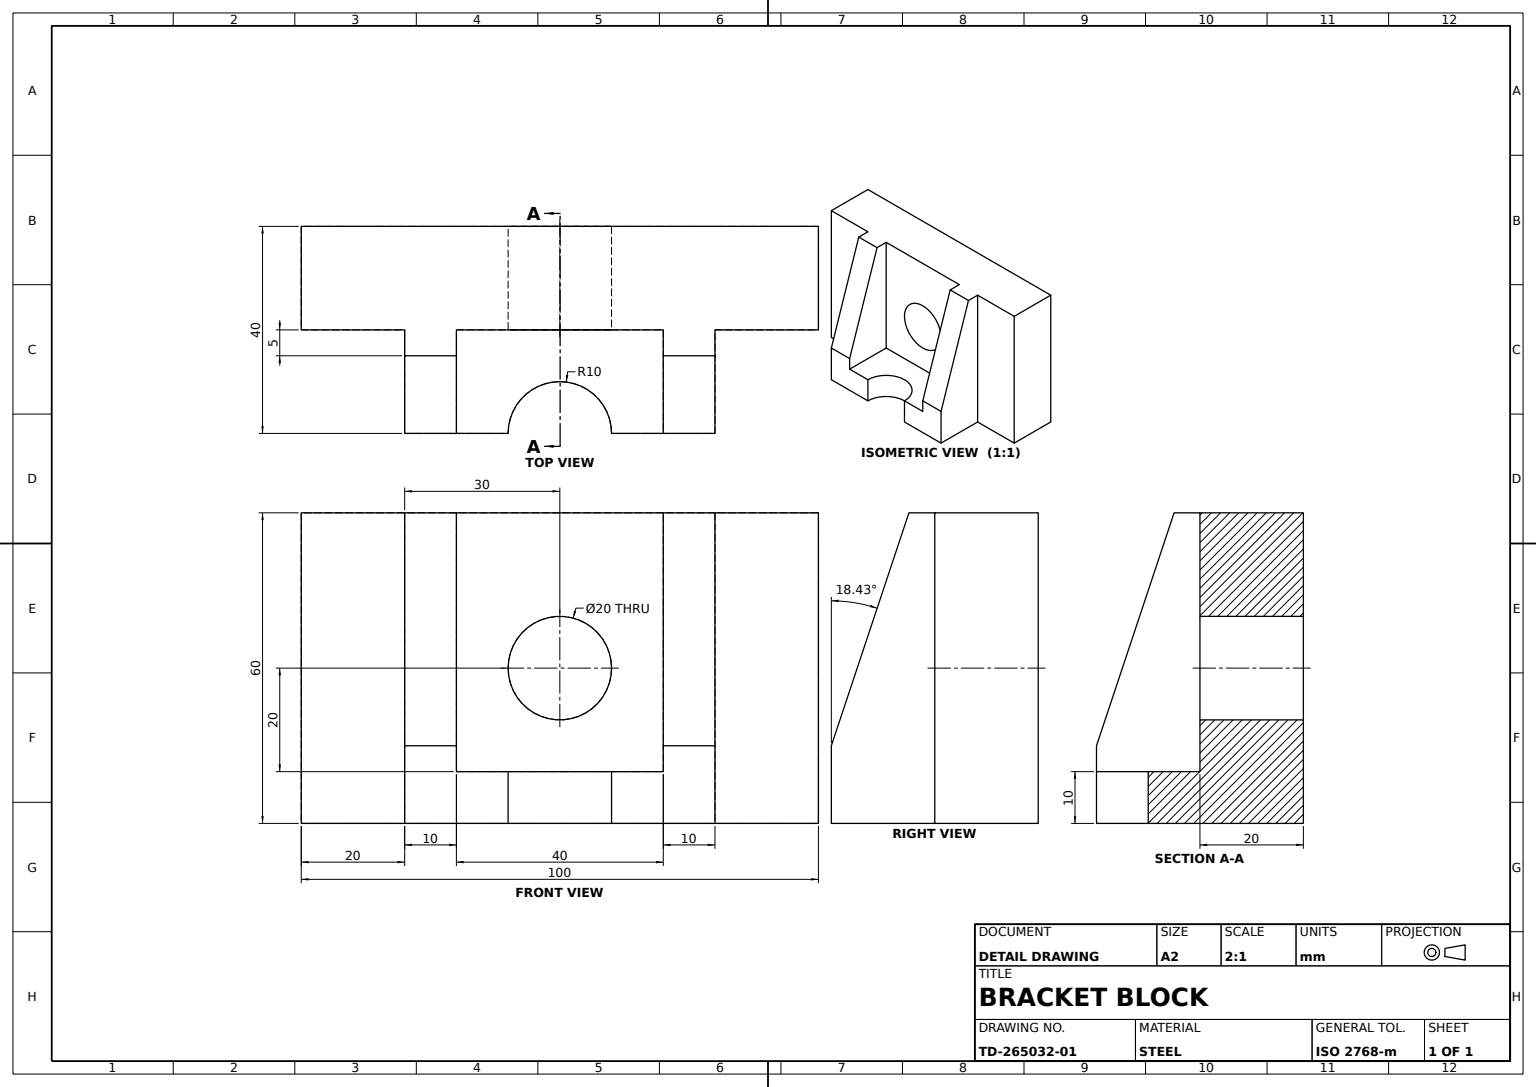
SolidWorks part; units mm, degrees
material "Plain Carbon Steel"
ref_plane "Front Plane" through (0, 0, 0) normal (0, 0, 1) x (1, 0, 0)
ref_plane "Top Plane" through (0, 0, 0) normal (0, 1, 0) x (1, 0, 0)
ref_plane "Right Plane" through (0, 0, 0) normal (1, 0, 0) x (0, 0, -1)
sketch "Back Plate Sketch" plane through (0, 0, 0) normal (0, 0, 1) x (1, 0, 0)
  line L0 (0, 0) -> (100, 0)
  line L1 (100, 0) -> (100, 60)
  line L2 (100, 60) -> (0, 60)
  line L3 (0, 60) -> (0, 0)
  dimension "D1" = 100
  dimension "D2" = 60
extrude "Back Plate" add sketch "Back Plate Sketch" along normal blind 20
sketch "Bore Ø20 Sketch" plane through (0, 0, 20) normal (0, 0, 1) x (1, 0, 0)
  line L0 (0, 60) -> (0, 0) construction
  line L1 (0, 0) -> (100, 0) construction
  circle A0 centre (50, 30) radius 10
  dimension "D1" = 20
  dimension "D2" = 20
  dimension "D3" = 50
  dimension "D4" = 30
extrude "Bore Ø20" cut sketch "Bore Ø20 Sketch" against normal blind 20
sketch "Base Flange Sketch" plane through (0, 0, 0) normal (0, -1, 0) x (1, 0, 0)
  line L0 (100, 20) -> (100, 0) construction
  line L1 (0, 20) -> (100, 20) construction
  line L2 (20, 20) -> (20, 40)
  line L3 (20, 40) -> (40, 40)
  line L5 (80, 20) -> (80, 40)
  line L6 (80, 40) -> (60, 40)
  line L7 (20, 20) -> (80, 20)
  arc A0 (40, 40) -> (60, 40) centre (50, 40) ccw
  dimension "D1" = 20
  dimension "D2" = 10
  dimension "D3" = 20
  dimension "D4" = 50
extrude "Notched Base Flange" add sketch "Base Flange Sketch" against normal blind 10
sketch "Left Gusset Sketch" plane through (80, 0, 0) normal (1, 0, 0) x (0, 0, -1)
  line L0 (-40, 10) -> (-40, 15)
  line L1 (-20, 60) -> (-25, 60)
  line L2 (-25, 60) -> (-40, 15)
  line L3 (-20, 60) -> (-20, 10)
  line L4 (-20, 10) -> (-40, 10)
  dimension "D1" = 5
extrude "Left Gusset" add sketch "Left Gusset Sketch" against normal blind 10
sketch "Right Gusset Sketch" plane through (20, 0, 0) normal (-1, 0, 0) x (0, 0, 1)
  line L0 (40, 10) -> (40, 15)
  line L1 (40, 15) -> (40, 10) construction
  line L2 (40, 15) -> (25, 60)
  line L3 (25, 60) -> (20, 60)
  line L4 (20, 60) -> (20, 10)
  line L5 (20, 10) -> (40, 10)
extrude "Right Gusset" add sketch "Right Gusset Sketch" against normal blind 10
